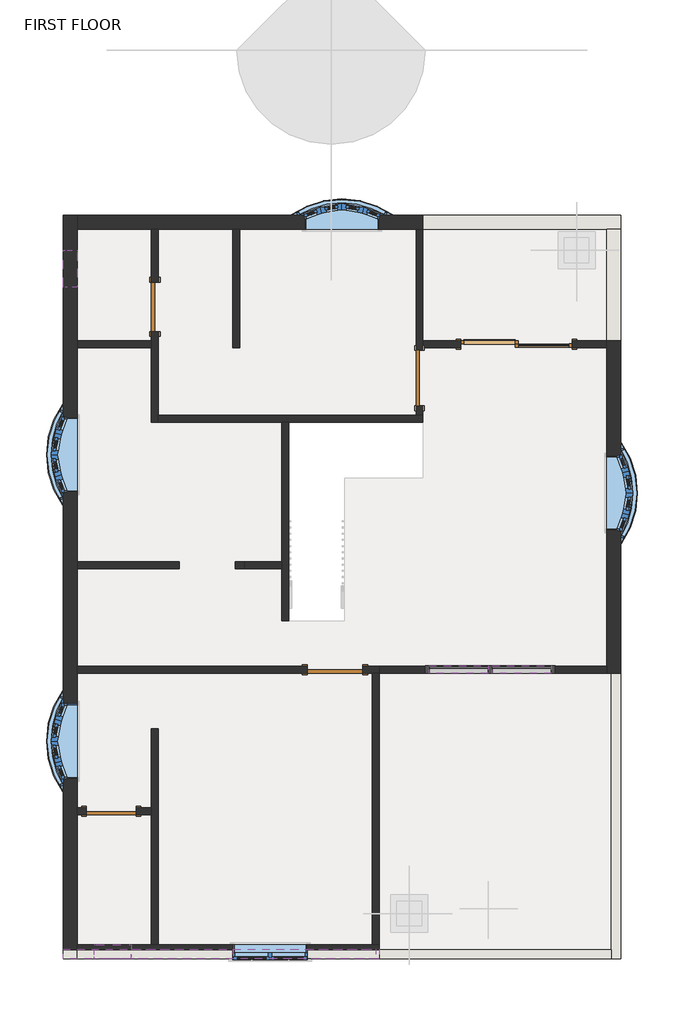
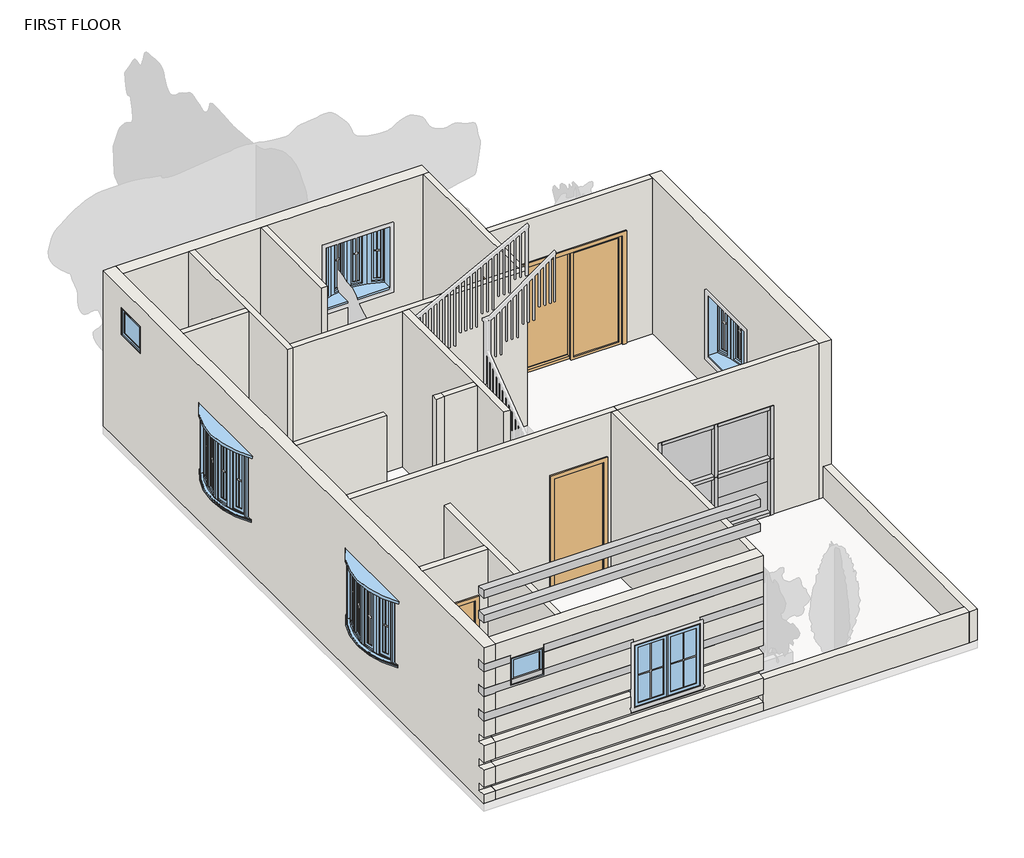
# One storey, part 1 of 2: 23 walls, 12 members, 7 windows, 5 doors, 5 plates, 5 proxies.
"""IFC4 building model written with IfcOpenShell, lengths in millimetres."""

from ifc_helpers import new_model, si_unit, frame, origin, place, context, project, spatial, polyline, outline, extrude, faceted_brep, transform, mapped, element, save
from components import door_166d4031, door_d141acb4, door_38851409, single_flush_3_x7_305aa2a5, single_flush_3_x7_310a3c6c, member_801a2072, member_e80433b6, member_309cb93c, member_88aa5c81, member_69c8e218, member_6ef8dc49, system_panel_glazed_3235cd3f, system_panel_glazed_537ed4da, system_panel_glazed_fc95d3d1, window_9e637e28, window_bow_casement_10_degree_angle_4_x4_fc1e5cf1, window_casement_double_4_x4_af3140d2

model = new_model("IFC4")

# Units and contexts
model_context = context("Model", 3, world=origin())
ifc_project = project(units=[si_unit("LENGTHUNIT", "METRE", prefix="MILLI")], contexts=[model_context])

# Site, building, storey
site = spatial("IfcSite", under=ifc_project)
building = spatial("IfcBuilding", under=site)
storey = spatial("IfcBuildingStorey", under=building, Name="FIRST FLOOR", Elevation=3200.4)

# Proxies
placement = place(None, origin())
element("IfcBuildingElementProxy", 1, Name="Reveal", ObjectType="Reveal", at=placement, inside=storey, context=model_context, shape_type="SweptSolid", body=[
    extrude(outline(polyline([(-5827.2415084, -5557.8064015), (-5827.2415084, -5405.4064015), (-702.7915084, -5405.4064015), (-702.7915084, -5557.8064015), (-5827.2415084, -5557.8064015)])), frame((0.0, 0.0, 7218.9473684), z_axis=(0.0, 0.0, 1.0), x_axis=(1.0, 0.0, 0.0)), (0.0, 0.0, 1.0), 152.4),
])
element("IfcBuildingElementProxy", 2, Name="Reveal", ObjectType="Reveal", at=placement, inside=storey, context=model_context, shape_type="SweptSolid", body=[
    extrude(outline(polyline([(-5827.2415084, -5557.8064015), (-5827.2415084, -5405.4064015), (-702.7915084, -5405.4064015), (-702.7915084, -5557.8064015), (-5827.2415084, -5557.8064015)])), frame((0.0, 0.0, 6737.6842105), z_axis=(0.0, 0.0, 1.0), x_axis=(1.0, 0.0, 0.0)), (0.0, 0.0, 1.0), 152.4),
])
element("IfcBuildingElementProxy", 3, Name="Reveal", ObjectType="Reveal", at=placement, inside=storey, context=model_context, shape_type="SweptSolid", body=[
    extrude(outline(polyline([(-4712.8165084, -5557.8064015), (-4712.8165084, -5405.4064015), (-645.6415084, -5405.4064015), (-645.6415084, -5557.8064015), (-4712.8165084, -5557.8064015)])), frame((0.0, 0.0, 5775.1578947), z_axis=(0.0, 0.0, 1.0), x_axis=(1.0, 0.0, 0.0)), (0.0, 0.0, 1.0), 152.4),
    extrude(outline(polyline([(-5827.2415084, -5557.8064015), (-5827.2415084, -5405.4064015), (-5322.4165084, -5405.4064015), (-5322.4165084, -5557.8064015), (-5827.2415084, -5557.8064015)])), frame((0.0, 0.0, 5775.1578947), z_axis=(0.0, 0.0, 1.0), x_axis=(1.0, 0.0, 0.0)), (0.0, 0.0, 1.0), 152.4),
])
element("IfcBuildingElementProxy", 4, Name="Reveal", ObjectType="Reveal", at=placement, inside=storey, context=model_context, shape_type="SweptSolid", body=[
    extrude(outline(polyline([(-1823.7720223, -5557.8064015), (-1823.7720223, -5405.4064015), (-645.6415084, -5405.4064015), (-645.6415084, -5557.8064015), (-1823.7720223, -5557.8064015)])), frame((0.0, 0.0, 5293.8947368), z_axis=(0.0, 0.0, 1.0), x_axis=(1.0, 0.0, 0.0)), (0.0, 0.0, 1.0), 152.4),
    extrude(outline(polyline([(-5827.2415084, -5557.8064015), (-5827.2415084, -5405.4064015), (-3042.9720223, -5405.4064015), (-3042.9720223, -5557.8064015), (-5827.2415084, -5557.8064015)])), frame((0.0, 0.0, 5293.8947368), z_axis=(0.0, 0.0, 1.0), x_axis=(1.0, 0.0, 0.0)), (0.0, 0.0, 1.0), 152.4),
])
element("IfcBuildingElementProxy", 5, Name="Reveal", ObjectType="Reveal", at=placement, inside=storey, context=model_context, shape_type="SweptSolid", body=[
    extrude(outline(polyline([(-1823.7720223, -5557.8064015), (-1823.7720223, -5405.4064015), (-645.6415084, -5405.4064015), (-645.6415084, -5557.8064015), (-1823.7720223, -5557.8064015)])), frame((0.0, 0.0, 4812.6315789), z_axis=(0.0, 0.0, 1.0), x_axis=(1.0, 0.0, 0.0)), (0.0, 0.0, 1.0), 152.4),
    extrude(outline(polyline([(-5827.2415084, -5557.8064015), (-5827.2415084, -5405.4064015), (-3042.9720223, -5405.4064015), (-3042.9720223, -5557.8064015), (-5827.2415084, -5557.8064015)])), frame((0.0, 0.0, 4812.6315789), z_axis=(0.0, 0.0, 1.0), x_axis=(1.0, 0.0, 0.0)), (0.0, 0.0, 1.0), 152.4),
])

# Doors
door_shape = door_166d4031(model_context)
element("IfcDoor", 6, ObjectType="Door-Double-Sliding : 72\" x 84\"", at=placement, inside=storey, context=model_context, shape_type="MappedRepresentation", body=[
    mapped(door_shape, transform((1608.6084916, 4392.6435985, 3200.4), x_axis=(1.0, 0.0, 0.0), y_axis=(0.0, 1.0, 0.0), z_axis=(0.0, 0.0, 1.0))),
])
door_2_shape = door_d141acb4(model_context)
element("IfcDoor", 7, ObjectType="Single-Flush : 2'8\"X7'", at=placement, inside=storey, context=model_context, shape_type="MappedRepresentation", body=[
    mapped(door_2_shape, transform((-5039.8415084, -3138.4564015, 3200.4), x_axis=(-1.0, 0.0, 0.0), y_axis=(0.0, -1.0, 0.0), z_axis=(0.0, 0.0, 1.0))),
])
door_3_shape = door_38851409(model_context)
element("IfcDoor", 8, ObjectType="Single-Flush : 2'8\"X7'", at=placement, inside=storey, context=model_context, shape_type="MappedRepresentation", body=[
    mapped(door_3_shape, transform((-4322.2915084, 5135.5935985, 3200.4), x_axis=(0.0, -1.0, 0.0), y_axis=(1.0, 0.0, 0.0), z_axis=(0.0, 0.0, 1.0))),
])
single_flush_3_x7_shape = single_flush_3_x7_305aa2a5(model_context)
element("IfcDoor", 9, ObjectType="Single-Flush : 3'X7'", at=placement, inside=storey, context=model_context, shape_type="MappedRepresentation", body=[
    mapped(single_flush_3_x7_shape, transform((-1369.5415084, -814.3564015, 3200.4), x_axis=(1.0, 0.0, 0.0), y_axis=(0.0, 1.0, 0.0), z_axis=(0.0, 0.0, 1.0))),
])
single_flush_3_x7_2_shape = single_flush_3_x7_310a3c6c(model_context)
element("IfcDoor", 10, ObjectType="Single-Flush : 3'X7'", at=placement, inside=storey, context=model_context, shape_type="MappedRepresentation", body=[
    mapped(single_flush_3_x7_2_shape, transform((14.7584916, 3967.1935985, 3200.4), x_axis=(0.0, -1.0, 0.0), y_axis=(1.0, 0.0, 0.0), z_axis=(0.0, 0.0, 1.0))),
])

# Members
member_shape = member_801a2072(model_context)
element("IfcMember", 11, ObjectType="Rectangular Mullion : 2.5\" x 5\" rectangular", at=placement, inside=storey, context=model_context, shape_type="MappedRepresentation", body=[
    mapped(member_shape, transform((2180.1084916, -814.3564015, 5334.0), x_axis=(0.0, 0.0, 1.0), y_axis=(0.0, -1.0, 0.0), z_axis=(1.0, 0.0, 0.0))),
])
element("IfcMember", 12, ObjectType="Rectangular Mullion : 2.5\" x 5\" rectangular", at=placement, inside=storey, context=model_context, shape_type="MappedRepresentation", body=[
    mapped(member_shape, transform((1145.0584916, -814.3564015, 5334.0), x_axis=(0.0, 0.0, 1.0), y_axis=(0.0, -1.0, 0.0), z_axis=(1.0, 0.0, 0.0))),
])
element("IfcMember", 13, ObjectType="Rectangular Mullion : 2.5\" x 5\" rectangular", at=placement, inside=storey, context=model_context, shape_type="MappedRepresentation", body=[
    mapped(member_shape, transform((173.5084916, -814.3564015, 3200.4), x_axis=(0.0, 0.0, -1.0), y_axis=(0.0, -1.0, 0.0), z_axis=(-1.0, 0.0, 0.0))),
])
element("IfcMember", 14, ObjectType="Rectangular Mullion : 2.5\" x 5\" rectangular", at=placement, inside=storey, context=model_context, shape_type="MappedRepresentation", body=[
    mapped(member_shape, transform((1208.5584916, -814.3564015, 3200.4), x_axis=(0.0, 0.0, -1.0), y_axis=(0.0, -1.0, 0.0), z_axis=(-1.0, 0.0, 0.0))),
])
member_2_shape = member_e80433b6(model_context)
element("IfcMember", 15, ObjectType="Rectangular Mullion : 2.5\" x 5\" rectangular", at=placement, inside=storey, context=model_context, shape_type="MappedRepresentation", body=[
    mapped(member_2_shape, transform((1176.8084916, -814.3564015, 3200.4), x_axis=(1.0, 0.0, 0.0), y_axis=(0.0, -1.0, 0.0), z_axis=(0.0, 0.0, -1.0))),
])
member_3_shape = member_309cb93c(model_context)
element("IfcMember", 16, ObjectType="Rectangular Mullion : 2.5\" x 5\" rectangular", at=placement, inside=storey, context=model_context, shape_type="MappedRepresentation", body=[
    mapped(member_3_shape, transform((1176.8084916, -814.3564015, 4298.95), x_axis=(1.0, 0.0, 0.0), y_axis=(0.0, -1.0, 0.0), z_axis=(0.0, 0.0, -1.0))),
])
member_4_shape = member_88aa5c81(model_context)
element("IfcMember", 17, ObjectType="Rectangular Mullion : 2.5\" x 5\" rectangular", at=placement, inside=storey, context=model_context, shape_type="MappedRepresentation", body=[
    mapped(member_4_shape, transform((1145.0584916, -814.3564015, 4298.95), x_axis=(0.0, 0.0, 1.0), y_axis=(0.0, -1.0, 0.0), z_axis=(1.0, 0.0, 0.0))),
])
element("IfcMember", 18, ObjectType="Rectangular Mullion : 2.5\" x 5\" rectangular", at=placement, inside=storey, context=model_context, shape_type="MappedRepresentation", body=[
    mapped(member_4_shape, transform((2180.1084916, -814.3564015, 4298.95), x_axis=(0.0, 0.0, 1.0), y_axis=(0.0, -1.0, 0.0), z_axis=(1.0, 0.0, 0.0))),
])
member_5_shape = member_69c8e218(model_context)
element("IfcMember", 19, ObjectType="Rectangular Mullion : 2.5\" x 5\" rectangular", at=placement, inside=storey, context=model_context, shape_type="MappedRepresentation", body=[
    mapped(member_5_shape, transform((2243.6084916, -814.3564015, 3200.4), x_axis=(1.0, 0.0, 0.0), y_axis=(0.0, -1.0, 0.0), z_axis=(0.0, 0.0, -1.0))),
])
member_6_shape = member_6ef8dc49(model_context)
element("IfcMember", 20, ObjectType="Rectangular Mullion : 2.5\" x 5\" rectangular", at=placement, inside=storey, context=model_context, shape_type="MappedRepresentation", body=[
    mapped(member_6_shape, transform((110.0084916, -814.3564015, 5334.0), x_axis=(-1.0, 0.0, 0.0), y_axis=(0.0, -1.0, 0.0), z_axis=(0.0, 0.0, 1.0))),
])
element("IfcMember", 21, ObjectType="Rectangular Mullion : 2.5\" x 5\" rectangular", at=placement, inside=storey, context=model_context, shape_type="MappedRepresentation", body=[
    mapped(member_5_shape, transform((110.0084916, -814.3564015, 4298.95), x_axis=(-1.0, 0.0, 0.0), y_axis=(0.0, -1.0, 0.0), z_axis=(0.0, 0.0, 1.0))),
])
element("IfcMember", 22, ObjectType="Rectangular Mullion : 2.5\" x 5\" rectangular", at=placement, inside=storey, context=model_context, shape_type="MappedRepresentation", body=[
    mapped(member_6_shape, transform((2243.6084916, -814.3564015, 4298.95), x_axis=(1.0, 0.0, 0.0), y_axis=(0.0, -1.0, 0.0), z_axis=(0.0, 0.0, -1.0))),
])

# Plates
system_panel_glazed_shape = system_panel_glazed_3235cd3f(model_context)
element("IfcPlate", 23, ObjectType="System Panel : Glazed", at=placement, inside=storey, context=model_context, shape_type="MappedRepresentation", body=[
    mapped(system_panel_glazed_shape, transform((1176.8084916, -814.3564015, 3200.4), x_axis=(1.0, 0.0, 0.0), y_axis=(0.0, 1.0, 0.0), z_axis=(0.0, 0.0, 1.0))),
])
system_panel_glazed_2_shape = system_panel_glazed_537ed4da(model_context)
element("IfcPlate", 24, ObjectType="System Panel : Glazed", at=placement, inside=storey, context=model_context, shape_type="MappedRepresentation", body=[
    mapped(system_panel_glazed_2_shape, transform((659.2834916, -814.3564015, 3263.9), x_axis=(1.0, 0.0, 0.0), y_axis=(0.0, 1.0, 0.0), z_axis=(0.0, 0.0, 1.0))),
])
element("IfcPlate", 25, ObjectType="System Panel : Glazed", at=placement, inside=storey, context=model_context, shape_type="MappedRepresentation", body=[
    mapped(system_panel_glazed_2_shape, transform((1694.3334916, -814.3564015, 3263.9), x_axis=(1.0, 0.0, 0.0), y_axis=(0.0, 1.0, 0.0), z_axis=(0.0, 0.0, 1.0))),
])
system_panel_glazed_3_shape = system_panel_glazed_fc95d3d1(model_context)
element("IfcPlate", 26, ObjectType="System Panel : Glazed", at=placement, inside=storey, context=model_context, shape_type="MappedRepresentation", body=[
    mapped(system_panel_glazed_3_shape, transform((659.2834916, -814.3564015, 4330.7), x_axis=(1.0, 0.0, 0.0), y_axis=(0.0, 1.0, 0.0), z_axis=(0.0, 0.0, 1.0))),
])
element("IfcPlate", 27, ObjectType="System Panel : Glazed", at=placement, inside=storey, context=model_context, shape_type="MappedRepresentation", body=[
    mapped(system_panel_glazed_3_shape, transform((1694.3334916, -814.3564015, 4330.7), x_axis=(1.0, 0.0, 0.0), y_axis=(0.0, 1.0, 0.0), z_axis=(0.0, 0.0, 1.0))),
])

# Walls
element("IfcWall", 28, ObjectType="4\"", at=placement, inside=storey, context=model_context, shape_type="Brep", body=[
    faceted_brep([(-36.0415084, 3509.9935985, 5334.0), (-36.0415084, 3509.9935985, 3200.4), (-36.0415084, 3357.5935985, 3200.4), (-36.0415084, 3357.5935985, 6248.4), (-36.0415084, 6405.5935985, 6248.4), (-36.0415084, 6405.5935985, 3200.4), (-36.0415084, 4424.3935985, 3200.4), (-36.0415084, 4424.3935985, 5334.0), (65.5584916, 3357.5935985, 3200.4), (65.5584916, 3509.9935985, 3200.4), (65.5584916, 3509.9935985, 5334.0), (65.5584916, 4424.3935985, 5334.0), (65.5584916, 4424.3935985, 3200.4), (65.5584916, 4462.4935985, 3200.4), (65.5584916, 4576.7935985, 3200.4), (65.5584916, 6405.5935985, 3200.4), (65.5584916, 6405.5935985, 6248.4), (65.5584916, 4576.7935985, 6248.4), (65.5584916, 4462.4935985, 6248.4), (65.5584916, 3357.5935985, 6248.4)], [[[0, 1, 2, 3, 4, 5, 6, 7]], [[8, 9, 10, 11, 12, 13, 14, 15, 16, 17, 18, 19]], [[6, 5, 15, 14, 13, 12]], [[2, 1, 9, 8]], [[4, 3, 19, 18, 17, 16]], [[3, 2, 8, 19]], [[10, 9, 1, 0]], [[11, 10, 0, 7]], [[12, 11, 7, 6]], [[4, 16, 15, 5]]]),
])
element("IfcWall", 29, ObjectType="4.5\"", at=placement, inside=storey, context=model_context, shape_type="Brep", body=[
    faceted_brep([(-912.3415084, -871.5064015, 5334.0), (-912.3415084, -871.5064015, 3200.4), (-759.9415084, -871.5064015, 3200.4), (-645.6415084, -871.5064015, 3200.4), (-645.6415084, -871.5064015, 6248.4), (-759.9415084, -871.5064015, 6248.4), (-5598.6415084, -871.5064015, 6248.4), (-5598.6415084, -871.5064015, 3200.4), (-1826.7415084, -871.5064015, 3200.4), (-1826.7415084, -871.5064015, 5334.0), (-645.6415084, -757.2064015, 3200.4), (-912.3415084, -757.2064015, 3200.4), (-912.3415084, -757.2064015, 5334.0), (-1826.7415084, -757.2064015, 5334.0), (-1826.7415084, -757.2064015, 3200.4), (-5598.6415084, -757.2064015, 3200.4), (-5598.6415084, -757.2064015, 6248.4), (-645.6415084, -757.2064015, 6248.4)], [[[0, 1, 2, 3, 4, 5, 6, 7, 8, 9]], [[10, 11, 12, 13, 14, 15, 16, 17]], [[8, 7, 15, 14]], [[3, 2, 1, 11, 10]], [[6, 5, 4, 17, 16]], [[7, 6, 16, 15]], [[4, 3, 10, 17]], [[12, 11, 1, 0]], [[13, 12, 0, 9]], [[14, 13, 9, 8]]]),
])
element("IfcWall", 30, ObjectType="4.5\"", at=placement, inside=storey, context=model_context, shape_type="SweptSolid", body=[
    extrude(outline(polyline([(-759.9415084, -5329.2064015), (-759.9415084, -871.5064015), (-645.6415084, -871.5064015), (-645.6415084, -5329.2064015), (-759.9415084, -5329.2064015)])), frame((0.0, 0.0, 3200.4), z_axis=(0.0, 0.0, 1.0), x_axis=(1.0, 0.0, 0.0)), (0.0, 0.0, 1.0), 3048.0),
])
element("IfcWall", 31, ObjectType="4.5\"", at=placement, inside=storey, context=model_context, shape_type="SweptSolid", body=[
    extrude(outline(polyline([(6248.4, 3088.1584916), (6248.4, -645.6415084), (3200.4, -645.6415084), (3200.4, 110.0084916), (5334.0, 110.0084916), (5334.0, 2243.6084916), (3200.4, 2243.6084916), (3200.4, 3088.1584916), (6248.4, 3088.1584916)])), frame((0.0, -871.5064015, 0.0), z_axis=(0.0, 1.0, 0.0), x_axis=(0.0, 0.0, 1.0)), (0.0, 0.0, 1.0), 114.3),
])
element("IfcWall", 32, ObjectType="4.5\"", at=placement, inside=storey, context=model_context, shape_type="SweptSolid", body=[
    extrude(outline(polyline([(5334.0, 2523.0084916), (3200.4, 2523.0084916), (3200.4, 3088.1584916), (6248.4, 3088.1584916), (6248.4, 65.5584916), (3200.4, 65.5584916), (3200.4, 694.2084916), (5334.0, 694.2084916), (5334.0, 2523.0084916)])), frame((0.0, 4462.4935985, 0.0), z_axis=(0.0, 1.0, 0.0), x_axis=(0.0, 0.0, 1.0)), (0.0, 0.0, 1.0), 114.3),
])
element("IfcWall", 33, ObjectType="4.5\"", at=placement, inside=storey, context=model_context, shape_type="SweptSolid", body=[
    extrude(outline(polyline([(-3045.9415084, 4462.4935985), (-3045.9415084, 6405.5935985), (-2931.6415084, 6405.5935985), (-2931.6415084, 4462.4935985), (-3045.9415084, 4462.4935985)])), frame((0.0, 0.0, 3200.4), z_axis=(0.0, 0.0, 1.0), x_axis=(1.0, 0.0, 0.0)), (0.0, 0.0, 1.0), 3048.0),
])
element("IfcWall", 34, ObjectType="4.5\"", at=placement, inside=storey, context=model_context, shape_type="Brep", body=[
    faceted_brep([(-4379.4415084, 4729.1935985, 5334.0), (-4379.4415084, 4729.1935985, 3200.4), (-4379.4415084, 4576.7935985, 3200.4), (-4379.4415084, 4462.4935985, 3200.4), (-4379.4415084, 3243.2935985, 3200.4), (-4379.4415084, 3243.2935985, 6248.4), (-4379.4415084, 4462.4935985, 6248.4), (-4379.4415084, 4576.7935985, 6248.4), (-4379.4415084, 6405.5935985, 6248.4), (-4379.4415084, 6405.5935985, 3200.4), (-4379.4415084, 5541.9935985, 3200.4), (-4379.4415084, 5541.9935985, 5334.0), (-4265.1415084, 3243.2935985, 3200.4), (-4265.1415084, 3357.5935985, 3200.4), (-4265.1415084, 4729.1935985, 3200.4), (-4265.1415084, 4729.1935985, 5334.0), (-4265.1415084, 5541.9935985, 5334.0), (-4265.1415084, 5541.9935985, 3200.4), (-4265.1415084, 6405.5935985, 3200.4), (-4265.1415084, 6405.5935985, 6248.4), (-4265.1415084, 3357.5935985, 6248.4), (-4265.1415084, 3243.2935985, 6248.4)], [[[0, 1, 2, 3, 4, 5, 6, 7, 8, 9, 10, 11]], [[12, 13, 14, 15, 16, 17, 18, 19, 20, 21]], [[10, 9, 18, 17]], [[4, 3, 2, 1, 14, 13, 12]], [[8, 7, 6, 5, 21, 20, 19]], [[9, 8, 19, 18]], [[5, 4, 12, 21]], [[15, 14, 1, 0]], [[16, 15, 0, 11]], [[17, 16, 11, 10]]]),
])
element("IfcWall", 35, ObjectType="4.5\"", at=placement, inside=storey, context=model_context, shape_type="SweptSolid", body=[
    extrude(outline(polyline([(-5598.6415084, 4576.7935985), (-4379.4415084, 4576.7935985), (-4379.4415084, 4462.4935985), (-5598.6415084, 4462.4935985), (-5598.6415084, 4576.7935985)])), frame((0.0, 0.0, 3200.4), z_axis=(0.0, 0.0, 1.0), x_axis=(1.0, 0.0, 0.0)), (0.0, 0.0, 1.0), 3048.0),
])
element("IfcWall", 36, ObjectType="4.5\"", at=placement, inside=storey, context=model_context, shape_type="Brep", body=[
    faceted_brep([(-4265.1415084, 3243.2935985, 3200.4), (-2245.8415084, 3243.2935985, 3200.4), (-2131.5415084, 3243.2935985, 3200.4), (65.5584916, 3243.2935985, 3200.4), (65.5584916, 3243.2935985, 6248.4), (-2131.5415084, 3243.2935985, 6248.4), (-2245.8415084, 3243.2935985, 6248.4), (-4265.1415084, 3243.2935985, 6248.4), (-4265.1415084, 3357.5935985, 3200.4), (-4265.1415084, 3357.5935985, 6248.4), (-36.0415084, 3357.5935985, 6248.4), (65.5584916, 3357.5935985, 6248.4), (65.5584916, 3357.5935985, 3200.4), (-36.0415084, 3357.5935985, 3200.4)], [[[0, 1, 2, 3, 4, 5, 6, 7]], [[8, 9, 10, 11, 12, 13]], [[3, 2, 1, 0, 8, 13, 12]], [[7, 6, 5, 4, 11, 10, 9]], [[0, 7, 9, 8]], [[4, 3, 12, 11]]]),
])
element("IfcWall", 37, ObjectType="4.5\"", at=placement, inside=storey, context=model_context, shape_type="SweptSolid", body=[
    extrude(outline(polyline([(-3922.2415084, 842.9935985), (-5598.6415084, 842.9935985), (-5598.6415084, 957.2935985), (-3922.2415084, 957.2935985), (-3922.2415084, 842.9935985)])), frame((0.0, 0.0, 3200.4), z_axis=(0.0, 0.0, 1.0), x_axis=(1.0, 0.0, 0.0)), (0.0, 0.0, 1.0), 3048.0),
])
element("IfcWall", 38, ObjectType="4.5\"", at=placement, inside=storey, context=model_context, shape_type="SweptSolid", body=[
    extrude(outline(polyline([(-3007.8415084, 957.2935985), (-2855.4415084, 957.2935985), (-2855.4415084, 842.9935985), (-3007.8415084, 842.9935985), (-3007.8415084, 957.2935985)])), frame((0.0, 0.0, 3200.4), z_axis=(0.0, 0.0, 1.0), x_axis=(1.0, 0.0, 0.0)), (0.0, 0.0, 1.0), 3048.0),
])
element("IfcWall", 39, ObjectType="4.5\"", at=placement, inside=storey, context=model_context, shape_type="Brep", body=[
    faceted_brep([(-2245.8415084, 3243.2935985, 3200.4), (-2245.8415084, 957.2935985, 3200.4), (-2245.8415084, 842.9935985, 3200.4), (-2245.8415084, -9.4533727, 3200.4), (-2245.8415084, -9.4533727, 6248.4), (-2245.8415084, 842.9935985, 6248.4), (-2245.8415084, 957.2935985, 6248.4), (-2245.8415084, 3243.2935985, 6248.4), (-2131.5415084, 3243.2935985, 3200.4), (-2131.5415084, 3243.2935985, 6248.4), (-2131.5415084, -9.4533727, 6248.4), (-2131.5415084, -9.4533727, 3200.4)], [[[0, 1, 2, 3, 4, 5, 6, 7]], [[8, 9, 10, 11]], [[3, 2, 1, 0, 8, 11]], [[4, 3, 11, 10]], [[7, 6, 5, 4, 10, 9]], [[0, 7, 9, 8]]]),
])
element("IfcWall", 40, ObjectType="4.5\"", at=placement, inside=storey, context=model_context, shape_type="SweptSolid", body=[
    extrude(outline(polyline([(-2245.8415084, 842.9935985), (-2855.4415084, 842.9935985), (-2855.4415084, 957.2935985), (-2245.8415084, 957.2935985), (-2245.8415084, 842.9935985)])), frame((0.0, 0.0, 3200.4), z_axis=(0.0, 0.0, 1.0), x_axis=(1.0, 0.0, 0.0)), (0.0, 0.0, 1.0), 3048.0),
])
element("IfcWall", 41, ObjectType="4.5\"", at=placement, inside=storey, context=model_context, shape_type="Brep", body=[
    faceted_brep([(-4265.1415084, -5329.2064015, 3200.4), (-4265.1415084, -1785.9064015, 3200.4), (-4265.1415084, -1785.9064015, 6248.4), (-4265.1415084, -5329.2064015, 6248.4), (-4379.4415084, -5329.2064015, 3200.4), (-4379.4415084, -5329.2064015, 6248.4), (-4379.4415084, -3195.6064015, 6248.4), (-4379.4415084, -3081.3064015, 6248.4), (-4379.4415084, -1785.9064015, 6248.4), (-4379.4415084, -1785.9064015, 3200.4), (-4379.4415084, -3081.3064015, 3200.4), (-4379.4415084, -3195.6064015, 3200.4)], [[[0, 1, 2, 3]], [[4, 5, 6, 7, 8, 9, 10, 11]], [[1, 0, 4, 11, 10, 9]], [[2, 1, 9, 8]], [[3, 2, 8, 7, 6, 5]], [[0, 3, 5, 4]]]),
])
element("IfcWall", 42, ObjectType="4.5\"", at=placement, inside=storey, context=model_context, shape_type="SweptSolid", body=[
    extrude(outline(polyline([(3200.4, -5598.6415084), (3200.4, -5446.2415084), (5334.0, -5446.2415084), (5334.0, -4633.4415084), (3200.4, -4633.4415084), (3200.4, -4379.4415084), (6248.4, -4379.4415084), (6248.4, -5598.6415084), (3200.4, -5598.6415084)])), frame((0.0, -3195.6064015, 0.0), z_axis=(0.0, 1.0, 0.0), x_axis=(0.0, 0.0, 1.0)), (0.0, 0.0, 1.0), 114.3),
])
element("IfcWall", 43, ObjectType="6\"", at=placement, inside=storey, context=model_context, shape_type="Brep", body=[
    faceted_brep([(3164.3584916, -871.5064015, 3200.4), (3164.3584916, -5405.4064015, 3200.4), (3164.3584916, -5557.8064015, 3200.4), (3164.3584916, -5557.8064015, 3810.0), (3164.3584916, -5405.4064015, 3810.0), (3164.3584916, -871.5064015, 3810.0), (3316.7584916, -871.5064015, 3200.4), (3316.7584916, -871.5064015, 3810.0), (3316.7584916, -5557.8064015, 3810.0), (3316.7584916, -5557.8064015, 3200.4)], [[[0, 1, 2, 3, 4, 5]], [[6, 7, 8, 9]], [[2, 1, 0, 6, 9]], [[5, 4, 3, 8, 7]], [[0, 5, 7, 6]], [[3, 2, 9, 8]]]),
])
element("IfcWall", 44, ObjectType="6\"", at=placement, inside=storey, context=model_context, shape_type="Brep", body=[
    faceted_brep([(3164.3584916, -5405.4064015, 3200.4), (-645.6415084, -5405.4064015, 3200.4), (-645.6415084, -5405.4064015, 3810.0), (3164.3584916, -5405.4064015, 3810.0), (3164.3584916, -5557.8064015, 3200.4), (3164.3584916, -5557.8064015, 3810.0), (-645.6415084, -5557.8064015, 3810.0), (-645.6415084, -5557.8064015, 3521.2421053), (-645.6415084, -5557.8064015, 3368.8421053), (-645.6415084, -5557.8064015, 3200.4)], [[[0, 1, 2, 3]], [[4, 5, 6, 7, 8, 9]], [[1, 0, 4, 9]], [[3, 2, 6, 5]], [[0, 3, 5, 4]], [[2, 1, 9, 8, 7, 6]]]),
])
element("IfcWall", 45, ObjectType="9\"", at=placement, inside=storey, context=model_context, shape_type="Brep", body=[
    faceted_brep([(-5827.2415084, 6634.1935985, 3200.4), (-5827.2415084, -5557.8064015, 3200.4), (-5827.2415084, -5557.8064015, 3368.8421053), (-5827.2415084, -5405.4064015, 3368.8421053), (-5827.2415084, -5405.4064015, 3521.2421053), (-5827.2415084, -5557.8064015, 3521.2421053), (-5827.2415084, -5557.8064015, 3850.1052632), (-5827.2415084, -5405.4064015, 3850.1052632), (-5827.2415084, -5405.4064015, 4002.5052632), (-5827.2415084, -5557.8064015, 4002.5052632), (-5827.2415084, -5557.8064015, 4331.3684211), (-5827.2415084, -5405.4064015, 4331.3684211), (-5827.2415084, -5405.4064015, 4483.7684211), (-5827.2415084, -5557.8064015, 4483.7684211), (-5827.2415084, -5557.8064015, 4812.6315789), (-5827.2415084, -5405.4064015, 4812.6315789), (-5827.2415084, -5405.4064015, 4965.0315789), (-5827.2415084, -5557.8064015, 4965.0315789), (-5827.2415084, -5557.8064015, 5293.8947368), (-5827.2415084, -5405.4064015, 5293.8947368), (-5827.2415084, -5405.4064015, 5446.2947368), (-5827.2415084, -5557.8064015, 5446.2947368), (-5827.2415084, -5557.8064015, 5775.1578947), (-5827.2415084, -5405.4064015, 5775.1578947), (-5827.2415084, -5405.4064015, 5927.5578947), (-5827.2415084, -5557.8064015, 5927.5578947), (-5827.2415084, -5557.8064015, 6248.4), (-5827.2415084, 6634.1935985, 6248.4), (-5827.2415084, 6062.6935985, 5334.0), (-5827.2415084, 6062.6935985, 5867.4), (-5827.2415084, 5453.0935985, 5867.4), (-5827.2415084, 5453.0935985, 5334.0), (-5827.2415084, -1354.6176736, 5464.1323709), (-5827.2415084, -2621.5978876, 5464.1323709), (-5827.2415084, -2621.5978876, 4194.1323709), (-5827.2415084, -1354.6176736, 4194.1323709), (-5827.2415084, 3342.0645075, 5464.1323709), (-5827.2415084, 2075.0842935, 5464.1323709), (-5827.2415084, 2075.0842935, 4194.1323709), (-5827.2415084, 3342.0645075, 4194.1323709), (-5598.6415084, -5557.8064015, 3200.4), (-5598.6415084, -5329.2064015, 3200.4), (-5598.6415084, -3195.6064015, 3200.4), (-5598.6415084, -3081.3064015, 3200.4), (-5598.6415084, -871.5064015, 3200.4), (-5598.6415084, -757.2064015, 3200.4), (-5598.6415084, 842.9935985, 3200.4), (-5598.6415084, 957.2935985, 3200.4), (-5598.6415084, 4462.4935985, 3200.4), (-5598.6415084, 4576.7935985, 3200.4), (-5598.6415084, 6405.5935985, 3200.4), (-5598.6415084, 6634.1935985, 3200.4), (-5598.6415084, 6634.1935985, 6248.4), (-5598.6415084, 6405.5935985, 6248.4), (-5598.6415084, 4576.7935985, 6248.4), (-5598.6415084, 4462.4935985, 6248.4), (-5598.6415084, 957.2935985, 6248.4), (-5598.6415084, 842.9935985, 6248.4), (-5598.6415084, -757.2064015, 6248.4), (-5598.6415084, -871.5064015, 6248.4), (-5598.6415084, -3081.3064015, 6248.4), (-5598.6415084, -3195.6064015, 6248.4), (-5598.6415084, -5329.2064015, 6248.4), (-5598.6415084, -5557.8064015, 6248.4), (-5598.6415084, -5557.8064015, 5927.5578947), (-5598.6415084, -5405.4064015, 5927.5578947), (-5598.6415084, -5405.4064015, 5775.1578947), (-5598.6415084, -5557.8064015, 5775.1578947), (-5598.6415084, -5557.8064015, 5446.2947368), (-5598.6415084, -5405.4064015, 5446.2947368), (-5598.6415084, -5405.4064015, 5293.8947368), (-5598.6415084, -5557.8064015, 5293.8947368), (-5598.6415084, -5557.8064015, 4965.0315789), (-5598.6415084, -5405.4064015, 4965.0315789), (-5598.6415084, -5405.4064015, 4812.6315789), (-5598.6415084, -5557.8064015, 4812.6315789), (-5598.6415084, -5557.8064015, 4483.7684211), (-5598.6415084, -5405.4064015, 4483.7684211), (-5598.6415084, -5405.4064015, 4331.3684211), (-5598.6415084, -5557.8064015, 4331.3684211), (-5598.6415084, -5557.8064015, 4002.5052632), (-5598.6415084, -5405.4064015, 4002.5052632), (-5598.6415084, -5405.4064015, 3850.1052632), (-5598.6415084, -5557.8064015, 3850.1052632), (-5598.6415084, -5557.8064015, 3521.2421053), (-5598.6415084, -5405.4064015, 3521.2421053), (-5598.6415084, -5405.4064015, 3368.8421053), (-5598.6415084, -5557.8064015, 3368.8421053), (-5598.6415084, 6062.6935985, 5867.4), (-5598.6415084, 6062.6935985, 5334.0), (-5598.6415084, 5453.0935985, 5334.0), (-5598.6415084, 5453.0935985, 5867.4), (-5598.6415084, -2597.7077806, 5464.1323709), (-5598.6415084, -1378.5077806, 5464.1323709), (-5598.6415084, -1378.5077806, 4194.1323709), (-5598.6415084, -2597.7077806, 4194.1323709), (-5598.6415084, 2098.9744005, 5464.1323709), (-5598.6415084, 3318.1744005, 5464.1323709), (-5598.6415084, 3318.1744005, 4194.1323709), (-5598.6415084, 2098.9744005, 4194.1323709), (-5761.6039788, -2597.7077806, 5464.1323709), (-5761.6039788, -1378.5077806, 5464.1323709), (-5761.6039788, -2597.7077806, 4194.1323709), (-5761.6039788, -1378.5077806, 4194.1323709), (-5761.6039788, 2098.9744005, 5464.1323709), (-5761.6039788, 3318.1744005, 5464.1323709), (-5761.6039788, 2098.9744005, 4194.1323709), (-5761.6039788, 3318.1744005, 4194.1323709)], [[[0, 1, 2, 3, 4, 5, 6, 7, 8, 9, 10, 11, 12, 13, 14, 15, 16, 17, 18, 19, 20, 21, 22, 23, 24, 25, 26, 27], [28, 29, 30, 31], [32, 33, 34, 35], [36, 37, 38, 39]], [[40, 41, 42, 43, 44, 45, 46, 47, 48, 49, 50, 51, 52, 53, 54, 55, 56, 57, 58, 59, 60, 61, 62, 63, 64, 65, 66, 67, 68, 69, 70, 71, 72, 73, 74, 75, 76, 77, 78, 79, 80, 81, 82, 83, 84, 85, 86, 87], [88, 89, 90, 91], [92, 93, 94, 95], [96, 97, 98, 99]], [[1, 0, 51, 50, 49, 48, 47, 46, 45, 44, 43, 42, 41, 40]], [[27, 26, 63, 62, 61, 60, 59, 58, 57, 56, 55, 54, 53, 52]], [[1, 40, 87, 2]], [[63, 26, 25, 64]], [[5, 84, 83, 6]], [[9, 80, 79, 10]], [[13, 76, 75, 14]], [[17, 72, 71, 18]], [[21, 68, 67, 22]], [[0, 27, 52, 51]], [[89, 88, 29, 28]], [[90, 89, 28, 31]], [[91, 90, 31, 30]], [[88, 91, 30, 29]], [[100, 33, 32, 101, 93, 92]], [[102, 95, 94, 103, 35, 34]], [[100, 92, 95, 102]], [[93, 101, 103, 94]], [[101, 32, 35, 103]], [[33, 100, 102, 34]], [[104, 37, 36, 105, 97, 96]], [[106, 99, 98, 107, 39, 38]], [[104, 96, 99, 106]], [[97, 105, 107, 98]], [[105, 36, 39, 107]], [[37, 104, 106, 38]], [[4, 85, 84, 5]], [[85, 4, 3, 86]], [[86, 3, 2, 87]], [[8, 81, 80, 9]], [[81, 8, 7, 82]], [[82, 7, 6, 83]], [[12, 77, 76, 13]], [[77, 12, 11, 78]], [[78, 11, 10, 79]], [[16, 73, 72, 17]], [[73, 16, 15, 74]], [[74, 15, 14, 75]], [[20, 69, 68, 21]], [[69, 20, 19, 70]], [[70, 19, 18, 71]], [[24, 65, 64, 25]], [[65, 24, 23, 66]], [[66, 23, 22, 67]]]),
])
element("IfcWall", 46, ObjectType="9\"", at=placement, inside=storey, context=model_context, shape_type="Brep", body=[
    faceted_brep([(-5598.6415084, -5557.8064015, 3200.4), (-645.6415084, -5557.8064015, 3200.4), (-645.6415084, -5557.8064015, 3368.8421053), (-5598.6415084, -5557.8064015, 3368.8421053), (-645.6415084, -5557.8064015, 6248.4), (-5598.6415084, -5557.8064015, 6248.4), (-5598.6415084, -5557.8064015, 5927.5578947), (-5322.4165084, -5557.8064015, 5927.5578947), (-5322.4165084, -5557.8064015, 5867.4), (-4712.8165084, -5557.8064015, 5867.4), (-4712.8165084, -5557.8064015, 5927.5578947), (-645.6415084, -5557.8064015, 5927.5578947), (-1823.7720223, -5557.8064015, 4114.8), (-3042.9720223, -5557.8064015, 4114.8), (-3042.9720223, -5557.8064015, 4331.3684211), (-5598.6415084, -5557.8064015, 4331.3684211), (-5598.6415084, -5557.8064015, 4002.5052632), (-645.6415084, -5557.8064015, 4002.5052632), (-645.6415084, -5557.8064015, 4331.3684211), (-1823.7720223, -5557.8064015, 4331.3684211), (-5598.6415084, -5557.8064015, 3521.2421053), (-645.6415084, -5557.8064015, 3521.2421053), (-645.6415084, -5557.8064015, 3810.0), (-645.6415084, -5557.8064015, 3850.1052632), (-5598.6415084, -5557.8064015, 3850.1052632), (-1823.7720223, -5557.8064015, 4483.7684211), (-645.6415084, -5557.8064015, 4483.7684211), (-645.6415084, -5557.8064015, 4812.6315789), (-1823.7720223, -5557.8064015, 4812.6315789), (-5598.6415084, -5557.8064015, 4483.7684211), (-3042.9720223, -5557.8064015, 4483.7684211), (-3042.9720223, -5557.8064015, 4812.6315789), (-5598.6415084, -5557.8064015, 4812.6315789), (-1823.7720223, -5557.8064015, 4965.0315789), (-645.6415084, -5557.8064015, 4965.0315789), (-645.6415084, -5557.8064015, 5293.8947368), (-1823.7720223, -5557.8064015, 5293.8947368), (-5598.6415084, -5557.8064015, 4965.0315789), (-3042.9720223, -5557.8064015, 4965.0315789), (-3042.9720223, -5557.8064015, 5293.8947368), (-5598.6415084, -5557.8064015, 5293.8947368), (-1823.7720223, -5557.8064015, 5334.0), (-1823.7720223, -5557.8064015, 5446.2947368), (-645.6415084, -5557.8064015, 5446.2947368), (-645.6415084, -5557.8064015, 5775.1578947), (-4712.8165084, -5557.8064015, 5775.1578947), (-4712.8165084, -5557.8064015, 5446.2947368), (-3042.9720223, -5557.8064015, 5446.2947368), (-3042.9720223, -5557.8064015, 5334.0), (-5598.6415084, -5557.8064015, 5446.2947368), (-5322.4165084, -5557.8064015, 5446.2947368), (-5322.4165084, -5557.8064015, 5775.1578947), (-5598.6415084, -5557.8064015, 5775.1578947), (-645.6415084, -5329.2064015, 3200.4), (-759.9415084, -5329.2064015, 3200.4), (-4265.1415084, -5329.2064015, 3200.4), (-4379.4415084, -5329.2064015, 3200.4), (-5598.6415084, -5329.2064015, 3200.4), (-5598.6415084, -5329.2064015, 6248.4), (-4379.4415084, -5329.2064015, 6248.4), (-4265.1415084, -5329.2064015, 6248.4), (-759.9415084, -5329.2064015, 6248.4), (-645.6415084, -5329.2064015, 6248.4), (-5322.4165084, -5329.2064015, 5867.4), (-5322.4165084, -5329.2064015, 5334.0), (-4712.8165084, -5329.2064015, 5334.0), (-4712.8165084, -5329.2064015, 5867.4), (-3042.9720223, -5329.2064015, 5334.0), (-3042.9720223, -5329.2064015, 4114.8), (-1823.7720223, -5329.2064015, 4114.8), (-1823.7720223, -5329.2064015, 5334.0), (-645.6415084, -5405.4064015, 3200.4), (-5598.6415084, -5405.4064015, 3368.8421053), (-5598.6415084, -5405.4064015, 3521.2421053), (-5598.6415084, -5405.4064015, 3850.1052632), (-5598.6415084, -5405.4064015, 4002.5052632), (-5598.6415084, -5405.4064015, 4331.3684211), (-5598.6415084, -5405.4064015, 4483.7684211), (-5598.6415084, -5405.4064015, 4812.6315789), (-5598.6415084, -5405.4064015, 4965.0315789), (-5598.6415084, -5405.4064015, 5293.8947368), (-5598.6415084, -5405.4064015, 5446.2947368), (-5598.6415084, -5405.4064015, 5775.1578947), (-5598.6415084, -5405.4064015, 5927.5578947), (-5322.4165084, -5405.4064015, 5867.4), (-5322.4165084, -5405.4064015, 5775.1578947), (-5322.4165084, -5405.4064015, 5446.2947368), (-5322.4165084, -5405.4064015, 5334.0), (-4712.8165084, -5405.4064015, 5334.0), (-4712.8165084, -5405.4064015, 5446.2947368), (-4712.8165084, -5405.4064015, 5775.1578947), (-4712.8165084, -5405.4064015, 5867.4), (-3042.9720223, -5405.4064015, 5334.0), (-3042.9720223, -5405.4064015, 5293.8947368), (-3042.9720223, -5405.4064015, 4965.0315789), (-3042.9720223, -5405.4064015, 4812.6315789), (-3042.9720223, -5405.4064015, 4483.7684211), (-3042.9720223, -5405.4064015, 4331.3684211), (-1823.7720223, -5405.4064015, 4331.3684211), (-1823.7720223, -5405.4064015, 4483.7684211), (-1823.7720223, -5405.4064015, 4812.6315789), (-1823.7720223, -5405.4064015, 4965.0315789), (-1823.7720223, -5405.4064015, 5293.8947368), (-1823.7720223, -5405.4064015, 5334.0), (-645.6415084, -5405.4064015, 5927.5578947), (-645.6415084, -5405.4064015, 5775.1578947), (-645.6415084, -5405.4064015, 5446.2947368), (-645.6415084, -5405.4064015, 5293.8947368), (-645.6415084, -5405.4064015, 4965.0315789), (-645.6415084, -5405.4064015, 4812.6315789), (-645.6415084, -5405.4064015, 4483.7684211), (-645.6415084, -5405.4064015, 4331.3684211), (-645.6415084, -5405.4064015, 4002.5052632), (-645.6415084, -5405.4064015, 3850.1052632), (-645.6415084, -5405.4064015, 3521.2421053), (-645.6415084, -5405.4064015, 3368.8421053), (-1823.7720223, -5405.4064015, 5446.2947368), (-3042.9720223, -5405.4064015, 5446.2947368), (-4712.8165084, -5405.4064015, 5927.5578947), (-5322.4165084, -5405.4064015, 5927.5578947)], [[[0, 1, 2, 3]], [[4, 5, 6, 7, 8, 9, 10, 11]], [[12, 13, 14, 15, 16, 17, 18, 19]], [[20, 21, 22, 23, 24]], [[25, 26, 27, 28]], [[29, 30, 31, 32]], [[33, 34, 35, 36]], [[37, 38, 39, 40]], [[41, 42, 43, 44, 45, 46, 47, 48]], [[49, 50, 51, 52]], [[53, 54, 55, 56, 57, 58, 59, 60, 61, 62], [63, 64, 65, 66], [67, 68, 69, 70]], [[1, 0, 57, 56, 55, 54, 53, 71]], [[5, 4, 62, 61, 60, 59, 58]], [[5, 58, 57, 0, 3, 72, 73, 20, 24, 74, 75, 16, 15, 76, 77, 29, 32, 78, 79, 37, 40, 80, 81, 49, 52, 82, 83, 6]], [[64, 63, 84, 85, 51, 50, 86, 87]], [[65, 64, 87, 88]], [[66, 65, 88, 89, 46, 45, 90, 91]], [[63, 66, 91, 9, 8, 84]], [[68, 67, 92, 93, 39, 38, 94, 95, 31, 30, 96, 97, 14, 13]], [[13, 12, 69, 68]], [[70, 69, 12, 19, 98, 99, 25, 28, 100, 101, 33, 36, 102, 103]], [[1, 71, 53, 62, 4, 11, 104, 105, 44, 43, 106, 107, 35, 34, 108, 109, 27, 26, 110, 111, 18, 17, 112, 113, 23, 22, 21, 114, 115, 2]], [[73, 114, 21, 20]], [[114, 73, 72, 115]], [[115, 72, 3, 2]], [[75, 112, 17, 16]], [[112, 75, 74, 113]], [[113, 74, 24, 23]], [[99, 110, 26, 25]], [[110, 99, 98, 111]], [[111, 98, 19, 18]], [[77, 96, 30, 29]], [[96, 77, 76, 97]], [[97, 76, 15, 14]], [[101, 108, 34, 33]], [[108, 101, 100, 109]], [[109, 100, 28, 27]], [[79, 94, 38, 37]], [[94, 79, 78, 95]], [[95, 78, 32, 31]], [[116, 42, 41, 103]], [[42, 116, 106, 43]], [[106, 116, 103, 102, 107]], [[107, 102, 36, 35]], [[47, 117, 92, 48]], [[117, 47, 46, 89]], [[81, 86, 50, 49]], [[86, 81, 80, 93, 92, 117, 89, 88, 87]], [[93, 80, 40, 39]], [[118, 10, 9, 91]], [[10, 118, 104, 11]], [[104, 118, 91, 90, 105]], [[105, 90, 45, 44]], [[7, 119, 84, 8]], [[119, 7, 6, 83]], [[84, 119, 83, 82, 85]], [[85, 82, 52, 51]], [[41, 48, 92, 67, 70, 103]]]),
])
element("IfcWall", 47, ObjectType="9\"", at=placement, inside=storey, context=model_context, shape_type="Brep", body=[
    faceted_brep([(3316.7584916, -871.5064015, 6248.4), (3316.7584916, -871.5064015, 3810.0), (3316.7584916, -871.5064015, 3200.4), (3316.7584916, 4576.7935985, 3200.4), (3316.7584916, 4576.7935985, 3810.0), (3316.7584916, 4576.7935985, 6248.4), (3316.7584916, 1447.7534915, 5080.0), (3316.7584916, 2714.7337055, 5080.0), (3316.7584916, 2714.7337055, 3810.0), (3316.7584916, 1447.7534915, 3810.0), (3088.1584916, -871.5064015, 3200.4), (3088.1584916, -871.5064015, 6248.4), (3088.1584916, -757.2064015, 6248.4), (3088.1584916, 4462.4935985, 6248.4), (3088.1584916, 4576.7935985, 6248.4), (3088.1584916, 4576.7935985, 3810.0), (3088.1584916, 4576.7935985, 3200.4), (3088.1584916, 4462.4935985, 3200.4), (3088.1584916, -757.2064015, 3200.4), (3088.1584916, 2690.8435985, 5080.0), (3088.1584916, 1471.6435985, 5080.0), (3088.1584916, 1471.6435985, 3810.0), (3088.1584916, 2690.8435985, 3810.0), (3164.3584916, -871.5064015, 3200.4), (3251.1209621, 2690.8435985, 5080.0), (3251.1209621, 1471.6435985, 5080.0), (3251.1209621, 2690.8435985, 3810.0), (3251.1209621, 1471.6435985, 3810.0)], [[[0, 1, 2, 3, 4, 5], [6, 7, 8, 9]], [[10, 11, 12, 13, 14, 15, 16, 17, 18], [19, 20, 21, 22]], [[3, 2, 23, 10, 18, 17, 16]], [[5, 4, 3, 16, 15, 14]], [[0, 5, 14, 13, 12, 11]], [[0, 11, 10, 23, 2, 1]], [[24, 7, 6, 25, 20, 19]], [[26, 22, 21, 27, 9, 8]], [[24, 19, 22, 26]], [[20, 25, 27, 21]], [[25, 6, 9, 27]], [[7, 24, 26, 8]]]),
])
element("IfcWall", 48, ObjectType="9\"", at=placement, inside=storey, context=model_context, shape_type="Brep", body=[
    faceted_brep([(65.5584916, 6634.1935985, 6248.4), (65.5584916, 6634.1935985, 3810.0), (65.5584916, 6634.1935985, 3200.4), (-5598.6415084, 6634.1935985, 3200.4), (-5598.6415084, 6634.1935985, 6248.4), (-621.7514014, 6634.1935985, 5464.1323709), (-1888.7316154, 6634.1935985, 5464.1323709), (-1888.7316154, 6634.1935985, 4194.1323709), (-621.7514014, 6634.1935985, 4194.1323709), (65.5584916, 6405.5935985, 3200.4), (65.5584916, 6405.5935985, 3810.0), (65.5584916, 6405.5935985, 6248.4), (-36.0415084, 6405.5935985, 6248.4), (-2931.6415084, 6405.5935985, 6248.4), (-3045.9415084, 6405.5935985, 6248.4), (-4265.1415084, 6405.5935985, 6248.4), (-4379.4415084, 6405.5935985, 6248.4), (-5598.6415084, 6405.5935985, 6248.4), (-5598.6415084, 6405.5935985, 3200.4), (-4379.4415084, 6405.5935985, 3200.4), (-4265.1415084, 6405.5935985, 3200.4), (-3045.9415084, 6405.5935985, 3200.4), (-2931.6415084, 6405.5935985, 3200.4), (-36.0415084, 6405.5935985, 3200.4), (-1864.8415084, 6405.5935985, 5464.1323709), (-645.6415084, 6405.5935985, 5464.1323709), (-645.6415084, 6405.5935985, 4194.1323709), (-1864.8415084, 6405.5935985, 4194.1323709), (-1864.8415084, 6568.5560689, 5464.1323709), (-645.6415084, 6568.5560689, 5464.1323709), (-1864.8415084, 6568.5560689, 4194.1323709), (-645.6415084, 6568.5560689, 4194.1323709)], [[[0, 1, 2, 3, 4], [5, 6, 7, 8]], [[9, 10, 11, 12, 13, 14, 15, 16, 17, 18, 19, 20, 21, 22, 23], [24, 25, 26, 27]], [[3, 2, 9, 23, 22, 21, 20, 19, 18]], [[0, 4, 17, 16, 15, 14, 13, 12, 11]], [[4, 3, 18, 17]], [[28, 6, 5, 29, 25, 24]], [[30, 27, 26, 31, 8, 7]], [[28, 24, 27, 30]], [[25, 29, 31, 26]], [[29, 5, 8, 31]], [[6, 28, 30, 7]], [[0, 11, 10, 9, 2, 1]]]),
])
element("IfcWall", 49, ObjectType="9\"", at=placement, inside=storey, context=model_context, shape_type="Brep", body=[
    faceted_brep([(65.5584916, 6405.5935985, 3200.4), (3088.1584916, 6405.5935985, 3200.4), (3316.7584916, 6405.5935985, 3200.4), (3316.7584916, 6405.5935985, 3810.0), (3088.1584916, 6405.5935985, 3810.0), (65.5584916, 6405.5935985, 3810.0), (65.5584916, 6634.1935985, 3200.4), (65.5584916, 6634.1935985, 3810.0), (3316.7584916, 6634.1935985, 3810.0), (3316.7584916, 6634.1935985, 3200.4)], [[[0, 1, 2, 3, 4, 5]], [[6, 7, 8, 9]], [[2, 1, 0, 6, 9]], [[5, 4, 3, 8, 7]], [[3, 2, 9, 8]], [[0, 5, 7, 6]]]),
])
element("IfcWall", 50, ObjectType="9\"", at=placement, inside=storey, context=model_context, shape_type="SweptSolid", body=[
    extrude(outline(polyline([(3088.1584916, 4576.7935985), (3088.1584916, 6405.5935985), (3316.7584916, 6405.5935985), (3316.7584916, 4576.7935985), (3088.1584916, 4576.7935985)])), frame((0.0, 0.0, 3200.4), z_axis=(0.0, 0.0, 1.0), x_axis=(1.0, 0.0, 0.0)), (0.0, 0.0, 1.0), 609.6),
])

# Windows
window_shape = window_9e637e28(model_context)
element("IfcWindow", 51, ObjectType="Fixed : 2'X1'9\"", at=placement, inside=storey, context=model_context, shape_type="MappedRepresentation", body=[
    mapped(window_shape, transform((-5055.7165084, -5443.5064015, 3200.4), x_axis=(-1.0, 0.0, 0.0), y_axis=(0.0, -1.0, 0.0), z_axis=(0.0, 0.0, 1.0))),
])
element("IfcWindow", 52, ObjectType="Fixed : 2'X1'9\"", at=placement, inside=storey, context=model_context, shape_type="MappedRepresentation", body=[
    mapped(window_shape, transform((-5712.9415084, 5795.9935985, 3200.4), x_axis=(0.0, 1.0, 0.0), y_axis=(-1.0, 0.0, 0.0), z_axis=(0.0, 0.0, 1.0))),
])
window_bow_casement_10_degree_angle_4_x4_shape = window_bow_casement_10_degree_angle_4_x4_fc1e5cf1(model_context)
element("IfcWindow", 53, ObjectType="Window-Bow-Casement-10_Degree_Angle : 4'X4'", at=placement, inside=storey, context=model_context, shape_type="MappedRepresentation", body=[
    mapped(window_bow_casement_10_degree_angle_4_x4_shape, transform((-5712.9415084, -1988.1077806, 3584.5323709), x_axis=(0.0, 1.0, 0.0), y_axis=(-1.0, 0.0, 0.0), z_axis=(0.0, 0.0, 1.0))),
])
element("IfcWindow", 54, ObjectType="Window-Bow-Casement-10_Degree_Angle : 4'X4'", at=placement, inside=storey, context=model_context, shape_type="MappedRepresentation", body=[
    mapped(window_bow_casement_10_degree_angle_4_x4_shape, transform((-5712.9415084, 2708.5744005, 3584.5323709), x_axis=(0.0, 1.0, 0.0), y_axis=(-1.0, 0.0, 0.0), z_axis=(0.0, 0.0, 1.0))),
])
element("IfcWindow", 55, ObjectType="Window-Bow-Casement-10_Degree_Angle : 4'X4'", at=placement, inside=storey, context=model_context, shape_type="MappedRepresentation", body=[
    mapped(window_bow_casement_10_degree_angle_4_x4_shape, transform((-1255.2415084, 6519.8935985, 3584.5323709), x_axis=(1.0, 0.0, 0.0), y_axis=(0.0, 1.0, 0.0), z_axis=(0.0, 0.0, 1.0))),
])
element("IfcWindow", 56, ObjectType="Window-Bow-Casement-10_Degree_Angle : 4'X4'", at=placement, inside=storey, context=model_context, shape_type="MappedRepresentation", body=[
    mapped(window_bow_casement_10_degree_angle_4_x4_shape, transform((3202.4584916, 2081.2435985, 3200.4), x_axis=(0.0, -1.0, 0.0), y_axis=(1.0, 0.0, 0.0), z_axis=(0.0, 0.0, 1.0))),
])
window_casement_double_4_x4_shape = window_casement_double_4_x4_af3140d2(model_context)
element("IfcWindow", 57, ObjectType="Window-Casement-Double : 4'X4'", at=placement, inside=storey, context=model_context, shape_type="MappedRepresentation", body=[
    mapped(window_casement_double_4_x4_shape, transform((-2433.3720223, -5443.5064015, 3200.4), x_axis=(-1.0, 0.0, 0.0), y_axis=(0.0, -1.0, 0.0), z_axis=(0.0, 0.0, 1.0))),
])

save(model, "model.ifc")

# Revit data of these elements
# Type "Door-Double-Sliding : 72\" x 84\""
#   Type Mark = "12"
#   Construction Type Id = "opn-d45"
#   Assembly Code = "C1020"
#   Analytic Construction = "Wood frame, double glass door "
#   Thickness = 0' - 2"
#   Thermal Resistance (R) = 1.8150 (h·ft²·°F)/BTU
#   Heat Transfer Coefficient (U) = 0.5510 BTU/(h·ft²·°F)
#   Height = 7' - 0"
#   Rail Width = 0' - 2"
#   Stiles = 0' - 2"
#   Trim Projection Ext = 0' - 1"
#   Trim Projection Int = 0' - 1"
#   Trim Width = 0' - 3"
#   Width = 6' - 0"
#   Define Thermal Properties by = 1
#   Glazing = Glass
#   Panel Material = Wood - Birch - Solid Stained Light Low Gloss
#   Trim Material = Paint - Sienna
#   Visual Light Transmittance = 0
#   Solar Heat Gain Coefficient = 0
#   Function = (empty or 0)
#   Wall Closure = (empty or 0)
# Type "Single-Flush : 2'8\"X7'"
#   Type Mark = "9"
#   Construction Type Id = "MDOOR"
#   Assembly Code = "C1020"
#   Analytic Construction = "Metal"
#   Thickness = 0' - 2"
#   Heat Transfer Coefficient (U) = 0.651978 BTU/(h·ft²·°F)
#   Height = 7' - 0"
#   Trim Projection Ext = 0' - 1"
#   Trim Projection Int = 0' - 1"
#   Trim Width = 0' - 3"
#   Width = 2' - 8"
#   Define Thermal Properties by = 1
#   Door Material = Door - Panel
#   Frame Material = Door - Frame
#   Visual Light Transmittance = 0
#   Solar Heat Gain Coefficient = 0
#   Function = (empty or 0)
#   Wall Closure = (empty or 0)
# Type "Single-Flush : 3'X7'"
#   Type Mark = "8"
#   Construction Type Id = "MDOOR"
#   Assembly Code = "C1020"
#   Analytic Construction = "Metal"
#   Thickness = 0' - 2"
#   Heat Transfer Coefficient (U) = 0.651978 BTU/(h·ft²·°F)
#   Height = 7' - 0"
#   Trim Projection Ext = 0' - 1"
#   Trim Projection Int = 0' - 1"
#   Trim Width = 0' - 3"
#   Width = 3' - 0"
#   Define Thermal Properties by = 1
#   Door Material = Door - Panel
#   Frame Material = Door - Frame
#   Visual Light Transmittance = 0
#   Solar Heat Gain Coefficient = 0
#   Function = (empty or 0)
#   Wall Closure = (empty or 0)
# Type "Rectangular Mullion : 2.5\" x 5\" rectangular"
#   built-in parameter 1007304 = 0.416667 (stored number, unit not read)
#   built-in parameter 1007301 = 0.104167 (stored number, unit not read)
#   built-in parameter 1007300 = 0.104167 (stored number, unit not read)
# Type "System Panel : Glazed"
#   Construction Type Id = "GSP4R"
#   Analytic Construction = "1/8 in Pilkington single glazing"
#   Visual Light Transmittance = 0.9
#   Solar Heat Gain Coefficient = 0.86
#   Heat Transfer Coefficient (U) = 1.18115 BTU/(h·ft²·°F)
#   Define Thermal Properties by = 1
# Type "4\""
#   Assembly Code = "B2010"
#   Layers, outside or top first: 0' - 4" no material (function 1)
# Type "4.5\""
#   Assembly Code = "B2010"
#   Layers, outside or top first: 0' - 4 1/2" no material (function 1)
# Type "6\""
#   Assembly Code = "B2010"
#   Layers, outside or top first: 0' - 6" "6\" wall" (function 1)
# Type "9\""
#   Assembly Code = "B2010"
#   Layers, outside or top first: 0' - 9" "wood" (function 1)
# Type "Fixed : 2'X1'9\""
#   Type Mark = "20"
#   Construction Type Id = "GSP4R"
#   Assembly Code = "B2020100"
#   Analytic Construction = "1/8 in Pilkington single glazing"
#   Visual Light Transmittance = 0.9
#   Solar Heat Gain Coefficient = 0.78
#   Heat Transfer Coefficient (U) = 0.6496 BTU/(h·ft²·°F)
#   Height = 1' - 9"
#   Default Sill Height = 7' - 0"
#   Width = 2' - 0"
#   Window Inset = 0' - 0 3/4"
#   Define Thermal Properties by = 1
#   Glass Pane Material = Glass
#   Sash Material = Sash
#   Wall Closure = (empty or 0)
# Type "Window-Bow-Casement-10_Degree_Angle : 4'X4'"
#   Type Mark = "27"
#   Fire Rating = "0.5h"
#   Assembly Code = "B2020100"
#   Analytic Construction = "Double glazing - domestic"
#   Width = 4' - 0"
#   Visual Light Transmittance = 0.81
#   Thermal Resistance (R) = 1.8146 (h·ft²·°F)/BTU
#   Solar Heat Gain Coefficient = 0.76
#   Rough Width = 4' - 0 1/2"
#   Rough Height = 4' - 0 1/2"
#   Radius 3 = 4' - 11.49333"
#   Radius 2 = 4' - 10.49333"
#   Radius 1 = 4' - 8.49333"
#   Length 7 = 4' - 9.19062"
#   Length 6 = 0' - 1.41593"
#   Length 5 = 1' - 1.00986"
#   Length 2 = 0' - 2.58415"
#   Depth 2 = 0' - 6.3557"
#   Length 4 = 0' - 1.03923"
#   Length 3 = 0' - 0.32476"
#   Length 1 = 0' - 10.27567"
#   Wall Thickness [instance default] = 0' - 6"
#   Trim Width = 4' - 4.64952"
#   Trim Height = 4' - 0"
#   Height 1 = 4' - 2"
#   Height = 4' - 0"
#   Heat Transfer Coefficient (U) = 0.5511 BTU/(h·ft²·°F)
#   Depth 1 = 0' - 5.29439"
#   Default Sill Height = 2' - 0"
#   Angle 2 = 15.00°
#   Angle 1 = 10.00°
#   Angle = 20.00°
#   Muntin Visibility = yes
#   Interior Trim Visibility [instance default] = yes
#   Exterior Trim Visibility [instance default] = yes
#   Muntin Pattern = Muntin Pattern_2x2 : Muntin Pattern_2x2
#   Interior Trim Material = Wood - Stained
#   Exterior Trim Material = Clad - White
#   Interior Trim = Trim-Window-Interior-Flat : Picture Frame
#   Interior Frame Material = Wood - Stained
#   Glass Panel Material = Glass
#   Exterior Frame Material = Clad - White
#   Wall Closure = (empty or 0)
# Type "Window-Casement-Double : 4'X4'"
#   Type Mark = "30"
#   Fire Rating = "0.5h"
#   Assembly Code = "B2020100"
#   Analytic Construction = "Double glazing - domestic"
#   Frame Extension [instance default] = 0' - 0 1/4"
#   Window Inset [instance default] = 0' - 0"
#   Wall Thickness [instance default] = 0' - 6"
#   Interior Wall Closure [instance default] = 0' - 2 1/4"
#   Half Width = 2' - 0"
#   Visual Light Transmittance = 0.81
#   Thermal Resistance (R) = 1.8146 (h·ft²·°F)/BTU
#   Solar Heat Gain Coefficient = 0.76
#   Rough Width = 4' - 0 1/2"
#   Rough Height = 4' - 0 1/2"
#   Height = 4' - 0"
#   Heat Transfer Coefficient (U) = 0.5511 BTU/(h·ft²·°F)
#   Exterior Wall Closure [instance default] = 0' - 1 1/4"
#   Extension Jamb [instance default] = 0' - 2 1/4"
#   Default Sill Height = 3' - 0"
#   Width = 4' - 0"
#   Muntin Visibility = yes
#   Interior Trim Visibility [instance default] = yes
#   Exterior Trim Visibility [instance default] = yes
#   Extension Jamb Visibility [instance default] = yes
#   Interior Trim Material = Wood - Stained
#   Muntin Pattern = Muntin Pattern_2x2 : Muntin Pattern_2x2
#   Interior Trim = Trim-Window-Interior-Flat : Picture Frame
#   Interior Frame Material = Wood - Stained
#   Glass Panel Material = Glass
#   Exterior Trim Material = Clad - White
#   Exterior Trim = Trim-Window-Exterior-Flat : with Sill
#   Exterior Frame Material = Clad - White
#   Wall Closure = (empty or 0)
# Element 6 (IfcDoor, "Door-Double-Sliding : 72\" x 84\"")
#   Phase Created = New Construction
#   Materials on its faces: "Paint - Sienna", "Wood - Birch - Solid Stained Light Low Gloss", "Glass"
# Elements 7, 8 (IfcDoor, "Single-Flush : 2'8\"X7'")
#   Phase Created = New Construction
#   Materials on its faces: "Door - Frame", "Door - Panel"
# Elements 9, 10 (IfcDoor, "Single-Flush : 3'X7'")
#   Phase Created = New Construction
#   Materials on its faces: "Door - Frame", "Door - Panel"
# Elements 11, 12, 13, 14, 15, 16, 17, 18, 19, 20, 21, 22 (IfcMember, "Rectangular Mullion : 2.5\" x 5\" rectangular")
#   Phase Created = New Construction
#   Materials on its faces: "Aluminum"
# Elements 23, 24, 25, 26, 27 (IfcPlate, "System Panel : Glazed")
#   Phase Created = New Construction
#   Materials on its faces: "Glass"
# Element 28 (IfcWall, "4\"")
#   Top Offset = -0' - 6"
#   Base Offset = 0' - 0"
#   wall height = 10' - 0"
#   Phase Created = New Construction
#   Base Constraint = FIRST FLOOR
#   Top Constraint = SECOND FLOOR
#   Materials on its faces: "Default Wall", "wall 1"
# Elements 29, 30, 31 (IfcWall, "4.5\"")
#   Top Offset = -0' - 6"
#   Base Offset = 0' - 0"
#   wall height = 10' - 0"
#   Phase Created = New Construction
#   Base Constraint = FIRST FLOOR
#   Top Constraint = SECOND FLOOR
#   Materials on its faces: "Default Wall", "wall 2"
# Elements 32, 36 (IfcWall, "4.5\"")
#   Top Offset = -0' - 6"
#   Base Offset = 0' - 0"
#   wall height = 10' - 0"
#   Phase Created = New Construction
#   Base Constraint = FIRST FLOOR
#   Top Constraint = SECOND FLOOR
#   Materials on its faces: "Default Wall", "wall 1"
# Elements 33, 34, 35, 37, 38, 39, 40, 41, 42 (IfcWall, "4.5\"")
#   Top Offset = -0' - 6"
#   Base Offset = 0' - 0"
#   wall height = 10' - 0"
#   Phase Created = New Construction
#   Base Constraint = FIRST FLOOR
#   Top Constraint = SECOND FLOOR
#   Materials on its faces: "Default Wall"
# Elements 43, 44 (IfcWall, "6\"")
#   Top Offset = -0' - 6"
#   Base Offset = 0' - 0"
#   Unconnected Height = 2' - 0"
#   wall height = 2' - 0"
#   Phase Created = New Construction
#   Base Constraint = FIRST FLOOR
#   Materials on its faces: "6\" wall"
# Elements 45, 46 (IfcWall, "9\"")
#   Top Offset = -0' - 6"
#   Base Offset = 0' - 0"
#   wall height = 10' - 0"
#   Phase Created = New Construction
